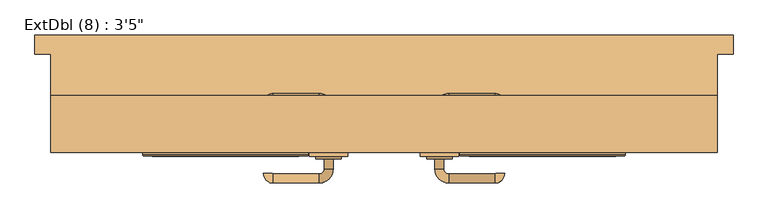
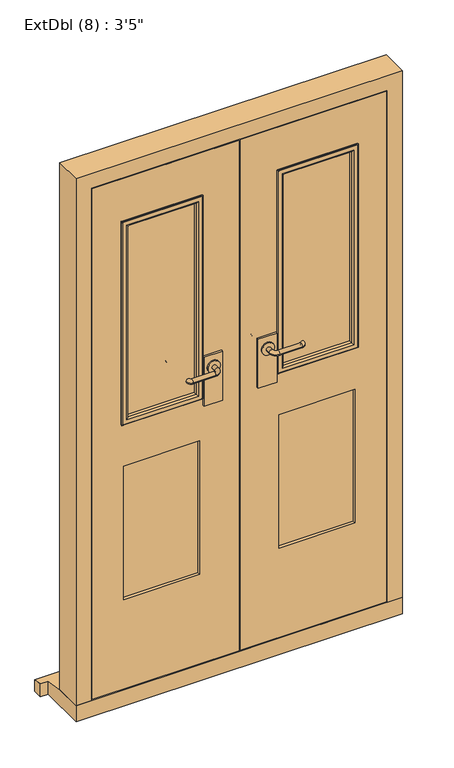
"""IFC4 building model written with IfcOpenShell, lengths in millimetres: door geometry."""

from ifc_helpers import new_model, si_unit, point, frame, frame_2d, origin, place, context, project, spatial, polyline, circle_curve, ellipse_curve, trimmed, segment, composite_curve, outline, extrude, faceted_brep, source, transform, mapped, element, save
from ifc_brep_helpers import plane_surface, cylinder_surface, revolved_surface, advanced_brep


def door_a196e7a2(model_context):
    return source(origin(), model_context, "Body", "SolidModel", [
        extrude(outline(composite_curve([segment(trimmed(circle_curve(frame_2d((1050.0, 86.5)), 20.0), [point((1050.0, 66.5))], [point((1050.0, 106.5))], False, "CARTESIAN"), True, "CONTINUOUS"), segment(trimmed(circle_curve(frame_2d((1050.0, 86.5)), 20.0), [point((1050.0, 106.5))], [point((1050.0, 66.5))], False, "CARTESIAN"), True, "CONTINUOUS")], self_intersect=False)), frame((0.0, -50.2929895, 0.0), z_axis=(0.0, 1.0, 0.0), x_axis=(0.0, 0.0, 1.0)), (0.0, 0.0, 1.0), 4.5929895),
        advanced_brep(
        [(93.5, -50.2929895, 1050.0), (79.5, -50.2929895, 1050.0), (79.5, -65.7, 1050.0), (93.5, -65.7, 1050.0), (101.5, -87.7, 1050.0), (101.5, -73.7, 1050.0), (173.5, -87.7, 1050.0), (173.5, -73.7, 1050.0), (174.5, -72.7, 1050.0), (188.5, -72.7, 1050.0)],
        [
            (0, 1, circle_curve(frame((86.5, -50.2929895, 1050.0), z_axis=(0.0, 1.0, 0.0), x_axis=(-1.0, 0.0, 0.0)), 7.0)),
            (1, 0, circle_curve(frame((86.5, -50.2929895, 1050.0), z_axis=(0.0, 1.0, 0.0), x_axis=(-1.0, 0.0, 0.0)), 7.0)),
            (1, 2),
            (2, 3, circle_curve(frame((86.5, -65.7, 1050.0), z_axis=(0.0, 1.0, 0.0), x_axis=(-1.0, 0.0, 0.0)), 7.0)),
            (3, 0),
            (3, 2, circle_curve(frame((86.5, -65.7, 1050.0), z_axis=(0.0, 1.0, 0.0), x_axis=(-1.0, 0.0, 0.0)), 7.0)),
            (4, 5, circle_curve(frame((101.5, -80.7, 1050.0), z_axis=(-1.0, 0.0, 0.0), x_axis=(0.0, -1.0, 0.0)), 7.0)),
            (5, 3, circle_curve(frame((101.5, -65.7, 1050.0), z_axis=(0.0, 0.0, -1.0), x_axis=(-1.0, 0.0, 0.0)), 8.0)),
            (2, 4, circle_curve(frame((101.5, -65.7, 1050.0), z_axis=(0.0, 0.0, 1.0), x_axis=(-1.0, 0.0, 0.0)), 22.0)),
            (5, 4, circle_curve(frame((101.5, -80.7, 1050.0), z_axis=(-1.0, 0.0, 0.0), x_axis=(0.0, -1.0, 0.0)), 7.0)),
            (4, 6),
            (6, 7, circle_curve(frame((173.5, -80.7, 1050.0), z_axis=(-1.0, 0.0, 0.0), x_axis=(0.0, -1.0, 0.0)), 7.0)),
            (7, 5),
            (7, 6, circle_curve(frame((173.5, -80.7, 1050.0), z_axis=(-1.0, 0.0, 0.0), x_axis=(0.0, -1.0, 0.0)), 7.0)),
            (8, 9, circle_curve(frame((181.5, -72.7, 1050.0), z_axis=(0.0, 1.0, 0.0), x_axis=(1.0, 0.0, 0.0)), 7.0)),
            (9, 8, circle_curve(frame((181.5, -72.7, 1050.0), z_axis=(0.0, 1.0, 0.0), x_axis=(1.0, 0.0, 0.0)), 7.0)),
            (8, 7, circle_curve(frame((173.5, -72.7, 1050.0), z_axis=(0.0, 0.0, -1.0), x_axis=(0.0, -1.0, 0.0)), 1.0)),
            (6, 9, circle_curve(frame((173.5, -72.7, 1050.0), z_axis=(0.0, 0.0, 1.0), x_axis=(0.0, -1.0, 0.0)), 15.0)),
        ],
        [
            plane_surface(frame((86.5, -50.2929895, 1050.0), z_axis=(0.0, 1.0, 0.0), x_axis=(0.0, 0.0, 1.0))),
            cylinder_surface(frame((86.5, -50.2929895, 1050.0), z_axis=(0.0, 1.0, 0.0), x_axis=(-1.0, 0.0, 0.0)), 7.0),
            revolved_surface(trimmed(ellipse_curve(frame((86.5, -65.7, 1050.0), z_axis=(0.0, -1.0, 0.0), x_axis=(-1.0, 0.0, 0.0)), 7.0, 7.0), [point((93.5, -65.7, 1050.0))], [point((79.5, -65.7, 1050.0))], True, "CARTESIAN"), (101.5, -65.7, 1050.0), (0.0, 0.0, -1.0)),
            revolved_surface(trimmed(ellipse_curve(frame((86.5, -65.7, 1050.0), z_axis=(0.0, -1.0, 0.0), x_axis=(-1.0, 0.0, 0.0)), 7.0, 7.0), [point((79.5, -65.7, 1050.0))], [point((93.5, -65.7, 1050.0))], True, "CARTESIAN"), (101.5, -65.7, 1050.0), (0.0, 0.0, -1.0)),
            cylinder_surface(frame((101.5, -80.7, 1050.0), z_axis=(-1.0, 0.0, 0.0), x_axis=(0.0, -1.0, 0.0)), 7.0),
            plane_surface(frame((181.5, -72.7, 1050.0), z_axis=(0.0, 1.0, 0.0), x_axis=(0.0, 0.0, 1.0))),
            revolved_surface(trimmed(ellipse_curve(frame((173.5, -80.7, 1050.0), z_axis=(1.0, 0.0, 0.0), x_axis=(0.0, -1.0, 0.0)), 7.0, 7.0), [point((173.5, -73.7, 1050.0))], [point((173.5, -87.7, 1050.0))], True, "CARTESIAN"), (173.5, -72.7, 1050.0), (0.0, 0.0, -1.0)),
            revolved_surface(trimmed(ellipse_curve(frame((173.5, -80.7, 1050.0), z_axis=(1.0, 0.0, 0.0), x_axis=(0.0, -1.0, 0.0)), 7.0, 7.0), [point((173.5, -87.7, 1050.0))], [point((173.5, -73.7, 1050.0))], True, "CARTESIAN"), (173.5, -72.7, 1050.0), (0.0, 0.0, -1.0)),
        ],
        [
            (0, [[1, 2]]),
            (1, [[3, 4, 5, -2]]),
            (1, [[-5, 6, -3, -1]]),
            (2, [[7, 8, -4, 9]]),
            (3, [[10, -9, -6, -8]]),
            (4, [[11, 12, 13, -7]]),
            (4, [[-13, 14, -11, -10]]),
            (5, [[15, 16]]),
            (6, [[-15, 17, -12, 18]]),
            (7, [[-16, -18, -14, -17]]),
        ],
    ),
        extrude(outline(polyline([(116.5, -39.7), (116.5, -45.7), (56.5, -45.7), (56.5, -39.7), (116.5, -39.7)])), frame((0.0, 0.0, 925.0), z_axis=(0.0, 0.0, 1.0), x_axis=(1.0, 0.0, 0.0)), (0.0, 0.0, 1.0), 165.0),
        extrude(outline(composite_curve([segment(trimmed(circle_curve(frame_2d((1050.0, -86.5)), 20.0), [point((1050.0, -66.5))], [point((1050.0, -106.5))], False, "CARTESIAN"), True, "CONTINUOUS"), segment(trimmed(circle_curve(frame_2d((1050.0, -86.5)), 20.0), [point((1050.0, -106.5))], [point((1050.0, -66.5))], False, "CARTESIAN"), True, "CONTINUOUS")], self_intersect=False)), frame((0.0, -50.2929895, 0.0), z_axis=(0.0, 1.0, 0.0), x_axis=(0.0, 0.0, 1.0)), (0.0, 0.0, 1.0), 4.5929895),
        advanced_brep(
        [(-93.5, -50.2929895, 1050.0), (-79.5, -50.2929895, 1050.0), (-93.5, -65.7, 1050.0), (-79.5, -65.7, 1050.0), (-101.5, -87.7, 1050.0), (-101.5, -73.7, 1050.0), (-173.5, -73.7, 1050.0), (-173.5, -87.7, 1050.0), (-174.5, -72.7, 1050.0), (-188.5, -72.7, 1050.0)],
        [
            (0, 1, circle_curve(frame((-86.5, -50.2929895, 1050.0), z_axis=(0.0, 1.0, 0.0), x_axis=(1.0, 0.0, 0.0)), 7.0)),
            (1, 0, circle_curve(frame((-86.5, -50.2929895, 1050.0), z_axis=(0.0, 1.0, 0.0), x_axis=(1.0, 0.0, 0.0)), 7.0)),
            (0, 2),
            (2, 3, circle_curve(frame((-86.5, -65.7, 1050.0), z_axis=(0.0, 1.0, 0.0), x_axis=(1.0, 0.0, 0.0)), 7.0)),
            (3, 1),
            (3, 2, circle_curve(frame((-86.5, -65.7, 1050.0), z_axis=(0.0, 1.0, 0.0), x_axis=(1.0, 0.0, 0.0)), 7.0)),
            (4, 3, circle_curve(frame((-101.5, -65.7, 1050.0), z_axis=(0.0, 0.0, 1.0), x_axis=(1.0, 0.0, 0.0)), 22.0)),
            (2, 5, circle_curve(frame((-101.5, -65.7, 1050.0), z_axis=(0.0, 0.0, -1.0), x_axis=(1.0, 0.0, 0.0)), 8.0)),
            (5, 4, circle_curve(frame((-101.5, -80.7, 1050.0), z_axis=(1.0, 0.0, 0.0), x_axis=(0.0, -1.0, 0.0)), 7.0)),
            (4, 5, circle_curve(frame((-101.5, -80.7, 1050.0), z_axis=(1.0, 0.0, 0.0), x_axis=(0.0, -1.0, 0.0)), 7.0)),
            (5, 6),
            (6, 7, circle_curve(frame((-173.5, -80.7, 1050.0), z_axis=(1.0, 0.0, 0.0), x_axis=(0.0, -1.0, 0.0)), 7.0)),
            (7, 4),
            (7, 6, circle_curve(frame((-173.5, -80.7, 1050.0), z_axis=(1.0, 0.0, 0.0), x_axis=(0.0, -1.0, 0.0)), 7.0)),
            (8, 9, circle_curve(frame((-181.5, -72.7, 1050.0), z_axis=(0.0, 1.0, 0.0), x_axis=(-1.0, 0.0, 0.0)), 7.0)),
            (9, 8, circle_curve(frame((-181.5, -72.7, 1050.0), z_axis=(0.0, 1.0, 0.0), x_axis=(-1.0, 0.0, 0.0)), 7.0)),
            (9, 7, circle_curve(frame((-173.5, -72.7, 1050.0), z_axis=(0.0, 0.0, 1.0), x_axis=(0.0, -1.0, 0.0)), 15.0)),
            (6, 8, circle_curve(frame((-173.5, -72.7, 1050.0), z_axis=(0.0, 0.0, -1.0), x_axis=(0.0, -1.0, 0.0)), 1.0)),
        ],
        [
            plane_surface(frame((-86.5, -50.2929895, 1050.0), z_axis=(0.0, 1.0, 0.0), x_axis=(0.0, 0.0, 1.0))),
            cylinder_surface(frame((-86.5, -50.2929895, 1050.0), z_axis=(0.0, 1.0, 0.0), x_axis=(1.0, 0.0, 0.0)), 7.0),
            revolved_surface(trimmed(ellipse_curve(frame((-86.5, -65.7, 1050.0), z_axis=(0.0, 1.0, 0.0), x_axis=(1.0, 0.0, 0.0)), 7.0, 7.0), [point((-93.5, -65.7, 1050.0))], [point((-79.5, -65.7, 1050.0))], True, "CARTESIAN"), (-101.5, -65.7, 1050.0), (0.0, 0.0, -1.0)),
            revolved_surface(trimmed(ellipse_curve(frame((-86.5, -65.7, 1050.0), z_axis=(0.0, 1.0, 0.0), x_axis=(1.0, 0.0, 0.0)), 7.0, 7.0), [point((-79.5, -65.7, 1050.0))], [point((-93.5, -65.7, 1050.0))], True, "CARTESIAN"), (-101.5, -65.7, 1050.0), (0.0, 0.0, -1.0)),
            cylinder_surface(frame((-101.5, -80.7, 1050.0), z_axis=(1.0, 0.0, 0.0), x_axis=(0.0, -1.0, 0.0)), 7.0),
            plane_surface(frame((-181.5, -72.7, 1050.0), z_axis=(0.0, 1.0, 0.0), x_axis=(0.0, 0.0, 1.0))),
            revolved_surface(trimmed(ellipse_curve(frame((-173.5, -80.7, 1050.0), z_axis=(1.0, 0.0, 0.0), x_axis=(0.0, -1.0, 0.0)), 7.0, 7.0), [point((-173.5, -73.7, 1050.0))], [point((-173.5, -87.7, 1050.0))], True, "CARTESIAN"), (-173.5, -72.7, 1050.0), (0.0, 0.0, -1.0)),
            revolved_surface(trimmed(ellipse_curve(frame((-173.5, -80.7, 1050.0), z_axis=(1.0, 0.0, 0.0), x_axis=(0.0, -1.0, 0.0)), 7.0, 7.0), [point((-173.5, -87.7, 1050.0))], [point((-173.5, -73.7, 1050.0))], True, "CARTESIAN"), (-173.5, -72.7, 1050.0), (0.0, 0.0, -1.0)),
        ],
        [
            (0, [[1, 2]]),
            (1, [[-1, 3, 4, 5]]),
            (1, [[-2, -5, 6, -3]]),
            (2, [[7, -4, 8, 9]]),
            (3, [[-8, -6, -7, 10]]),
            (4, [[-9, 11, 12, 13]]),
            (4, [[-10, -13, 14, -11]]),
            (5, [[15, 16]]),
            (6, [[17, -12, 18, -16]]),
            (7, [[-18, -14, -17, -15]]),
        ],
    ),
        extrude(outline(polyline([(-116.5, -39.7), (-56.5, -39.7), (-56.5, -45.7), (-116.5, -45.7), (-116.5, -39.7)])), frame((0.0, 0.0, 925.0), z_axis=(0.0, 0.0, 1.0), x_axis=(1.0, 0.0, 0.0)), (0.0, 0.0, 1.0), 165.0),
        extrude(outline(composite_curve([segment(trimmed(circle_curve(frame_2d((1050.0, -86.5)), 20.0), [point((1050.0, -66.5))], [point((1050.0, -106.5))], False, "CARTESIAN"), True, "CONTINUOUS"), segment(trimmed(circle_curve(frame_2d((1050.0, -86.5)), 20.0), [point((1050.0, -106.5))], [point((1050.0, -66.5))], False, "CARTESIAN"), True, "CONTINUOUS")], self_intersect=False)), frame((0.0, 10.3, 0.0), z_axis=(0.0, 1.0, 0.0), x_axis=(0.0, 0.0, 1.0)), (0.0, 0.0, 1.0), 4.5929895),
        advanced_brep(
        [(-93.5, 14.8929895, 1050.0), (-79.5, 14.8929895, 1050.0), (-79.5, 30.3, 1050.0), (-93.5, 30.3, 1050.0), (-101.5, 52.3, 1050.0), (-101.5, 38.3, 1050.0), (-173.5, 52.3, 1050.0), (-173.5, 38.3, 1050.0), (-174.5, 37.3, 1050.0), (-188.5, 37.3, 1050.0)],
        [
            (0, 1, circle_curve(frame((-86.5, 14.8929895, 1050.0), z_axis=(0.0, -1.0, 0.0), x_axis=(1.0, 0.0, 0.0)), 7.0)),
            (1, 0, circle_curve(frame((-86.5, 14.8929895, 1050.0), z_axis=(0.0, -1.0, 0.0), x_axis=(1.0, 0.0, 0.0)), 7.0)),
            (1, 2),
            (2, 3, circle_curve(frame((-86.5, 30.3, 1050.0), z_axis=(0.0, -1.0, 0.0), x_axis=(1.0, 0.0, 0.0)), 7.0)),
            (3, 0),
            (3, 2, circle_curve(frame((-86.5, 30.3, 1050.0), z_axis=(0.0, -1.0, 0.0), x_axis=(1.0, 0.0, 0.0)), 7.0)),
            (4, 5, circle_curve(frame((-101.5, 45.3, 1050.0), z_axis=(1.0, 0.0, 0.0), x_axis=(0.0, 1.0, 0.0)), 7.0)),
            (5, 3, circle_curve(frame((-101.5, 30.3, 1050.0), z_axis=(0.0, 0.0, -1.0), x_axis=(1.0, 0.0, 0.0)), 8.0)),
            (2, 4, circle_curve(frame((-101.5, 30.3, 1050.0), z_axis=(0.0, 0.0, 1.0), x_axis=(1.0, 0.0, 0.0)), 22.0)),
            (5, 4, circle_curve(frame((-101.5, 45.3, 1050.0), z_axis=(1.0, 0.0, 0.0), x_axis=(0.0, 1.0, 0.0)), 7.0)),
            (4, 6),
            (6, 7, circle_curve(frame((-173.5, 45.3, 1050.0), z_axis=(1.0, 0.0, 0.0), x_axis=(0.0, 1.0, 0.0)), 7.0)),
            (7, 5),
            (7, 6, circle_curve(frame((-173.5, 45.3, 1050.0), z_axis=(1.0, 0.0, 0.0), x_axis=(0.0, 1.0, 0.0)), 7.0)),
            (8, 9, circle_curve(frame((-181.5, 37.3, 1050.0), z_axis=(0.0, -1.0, 0.0), x_axis=(-1.0, 0.0, 0.0)), 7.0)),
            (9, 8, circle_curve(frame((-181.5, 37.3, 1050.0), z_axis=(0.0, -1.0, 0.0), x_axis=(-1.0, 0.0, 0.0)), 7.0)),
            (8, 7, circle_curve(frame((-173.5, 37.3, 1050.0), z_axis=(0.0, 0.0, -1.0), x_axis=(0.0, 1.0, 0.0)), 1.0)),
            (6, 9, circle_curve(frame((-173.5, 37.3, 1050.0), z_axis=(0.0, 0.0, 1.0), x_axis=(0.0, 1.0, 0.0)), 15.0)),
        ],
        [
            plane_surface(frame((-86.5, 14.8929895, 1050.0), z_axis=(0.0, -1.0, 0.0), x_axis=(0.0, 0.0, 1.0))),
            cylinder_surface(frame((-86.5, 14.8929895, 1050.0), z_axis=(0.0, -1.0, 0.0), x_axis=(1.0, 0.0, 0.0)), 7.0),
            revolved_surface(trimmed(ellipse_curve(frame((-86.5, 30.3, 1050.0), z_axis=(0.0, 1.0, 0.0), x_axis=(1.0, 0.0, 0.0)), 7.0, 7.0), [point((-93.5, 30.3, 1050.0))], [point((-79.5, 30.3, 1050.0))], True, "CARTESIAN"), (-101.5, 30.3, 1050.0), (0.0, 0.0, -1.0)),
            revolved_surface(trimmed(ellipse_curve(frame((-86.5, 30.3, 1050.0), z_axis=(0.0, 1.0, 0.0), x_axis=(1.0, 0.0, 0.0)), 7.0, 7.0), [point((-79.5, 30.3, 1050.0))], [point((-93.5, 30.3, 1050.0))], True, "CARTESIAN"), (-101.5, 30.3, 1050.0), (0.0, 0.0, -1.0)),
            cylinder_surface(frame((-101.5, 45.3, 1050.0), z_axis=(1.0, 0.0, 0.0), x_axis=(0.0, 1.0, 0.0)), 7.0),
            plane_surface(frame((-181.5, 37.3, 1050.0), z_axis=(0.0, -1.0, 0.0), x_axis=(0.0, 0.0, 1.0))),
            revolved_surface(trimmed(ellipse_curve(frame((-173.5, 45.3, 1050.0), z_axis=(-1.0, 0.0, 0.0), x_axis=(0.0, 1.0, 0.0)), 7.0, 7.0), [point((-173.5, 38.3, 1050.0))], [point((-173.5, 52.3, 1050.0))], True, "CARTESIAN"), (-173.5, 37.3, 1050.0), (0.0, 0.0, -1.0)),
            revolved_surface(trimmed(ellipse_curve(frame((-173.5, 45.3, 1050.0), z_axis=(-1.0, 0.0, 0.0), x_axis=(0.0, 1.0, 0.0)), 7.0, 7.0), [point((-173.5, 52.3, 1050.0))], [point((-173.5, 38.3, 1050.0))], True, "CARTESIAN"), (-173.5, 37.3, 1050.0), (0.0, 0.0, -1.0)),
        ],
        [
            (0, [[1, 2]]),
            (1, [[3, 4, 5, -2]]),
            (1, [[-5, 6, -3, -1]]),
            (2, [[7, 8, -4, 9]]),
            (3, [[10, -9, -6, -8]]),
            (4, [[11, 12, 13, -7]]),
            (4, [[-13, 14, -11, -10]]),
            (5, [[15, 16]]),
            (6, [[-15, 17, -12, 18]]),
            (7, [[-16, -18, -14, -17]]),
        ],
    ),
        extrude(outline(polyline([(-116.5, 4.3), (-116.5, 10.3), (-56.5, 10.3), (-56.5, 4.3), (-116.5, 4.3)])), frame((0.0, 0.0, 925.0), z_axis=(0.0, 0.0, 1.0), x_axis=(1.0, 0.0, 0.0)), (0.0, 0.0, 1.0), 165.0),
        extrude(outline(composite_curve([segment(trimmed(circle_curve(frame_2d((1050.0, 86.5)), 20.0), [point((1050.0, 66.5))], [point((1050.0, 106.5))], False, "CARTESIAN"), True, "CONTINUOUS"), segment(trimmed(circle_curve(frame_2d((1050.0, 86.5)), 20.0), [point((1050.0, 106.5))], [point((1050.0, 66.5))], False, "CARTESIAN"), True, "CONTINUOUS")], self_intersect=False)), frame((0.0, 10.3, 0.0), z_axis=(0.0, 1.0, 0.0), x_axis=(0.0, 0.0, 1.0)), (0.0, 0.0, 1.0), 4.5929895),
        advanced_brep(
        [(93.5, 14.8929895, 1050.0), (79.5, 14.8929895, 1050.0), (93.5, 30.3, 1050.0), (79.5, 30.3, 1050.0), (101.5, 52.3, 1050.0), (101.5, 38.3, 1050.0), (173.5, 38.3, 1050.0), (173.5, 52.3, 1050.0), (174.5, 37.3, 1050.0), (188.5, 37.3, 1050.0)],
        [
            (0, 1, circle_curve(frame((86.5, 14.8929895, 1050.0), z_axis=(0.0, -1.0, 0.0), x_axis=(-1.0, 0.0, 0.0)), 7.0)),
            (1, 0, circle_curve(frame((86.5, 14.8929895, 1050.0), z_axis=(0.0, -1.0, 0.0), x_axis=(-1.0, 0.0, 0.0)), 7.0)),
            (0, 2),
            (2, 3, circle_curve(frame((86.5, 30.3, 1050.0), z_axis=(0.0, -1.0, 0.0), x_axis=(-1.0, 0.0, 0.0)), 7.0)),
            (3, 1),
            (3, 2, circle_curve(frame((86.5, 30.3, 1050.0), z_axis=(0.0, -1.0, 0.0), x_axis=(-1.0, 0.0, 0.0)), 7.0)),
            (4, 3, circle_curve(frame((101.5, 30.3, 1050.0), z_axis=(0.0, 0.0, 1.0), x_axis=(-1.0, 0.0, 0.0)), 22.0)),
            (2, 5, circle_curve(frame((101.5, 30.3, 1050.0), z_axis=(0.0, 0.0, -1.0), x_axis=(-1.0, 0.0, 0.0)), 8.0)),
            (5, 4, circle_curve(frame((101.5, 45.3, 1050.0), z_axis=(-1.0, 0.0, 0.0), x_axis=(0.0, 1.0, 0.0)), 7.0)),
            (4, 5, circle_curve(frame((101.5, 45.3, 1050.0), z_axis=(-1.0, 0.0, 0.0), x_axis=(0.0, 1.0, 0.0)), 7.0)),
            (5, 6),
            (6, 7, circle_curve(frame((173.5, 45.3, 1050.0), z_axis=(-1.0, 0.0, 0.0), x_axis=(0.0, 1.0, 0.0)), 7.0)),
            (7, 4),
            (7, 6, circle_curve(frame((173.5, 45.3, 1050.0), z_axis=(-1.0, 0.0, 0.0), x_axis=(0.0, 1.0, 0.0)), 7.0)),
            (8, 9, circle_curve(frame((181.5, 37.3, 1050.0), z_axis=(0.0, -1.0, 0.0), x_axis=(1.0, 0.0, 0.0)), 7.0)),
            (9, 8, circle_curve(frame((181.5, 37.3, 1050.0), z_axis=(0.0, -1.0, 0.0), x_axis=(1.0, 0.0, 0.0)), 7.0)),
            (9, 7, circle_curve(frame((173.5, 37.3, 1050.0), z_axis=(0.0, 0.0, 1.0), x_axis=(0.0, 1.0, 0.0)), 15.0)),
            (6, 8, circle_curve(frame((173.5, 37.3, 1050.0), z_axis=(0.0, 0.0, -1.0), x_axis=(0.0, 1.0, 0.0)), 1.0)),
        ],
        [
            plane_surface(frame((86.5, 14.8929895, 1050.0), z_axis=(0.0, -1.0, 0.0), x_axis=(0.0, 0.0, 1.0))),
            cylinder_surface(frame((86.5, 14.8929895, 1050.0), z_axis=(0.0, -1.0, 0.0), x_axis=(-1.0, 0.0, 0.0)), 7.0),
            revolved_surface(trimmed(ellipse_curve(frame((86.5, 30.3, 1050.0), z_axis=(0.0, -1.0, 0.0), x_axis=(-1.0, 0.0, 0.0)), 7.0, 7.0), [point((93.5, 30.3, 1050.0))], [point((79.5, 30.3, 1050.0))], True, "CARTESIAN"), (101.5, 30.3, 1050.0), (0.0, 0.0, -1.0)),
            revolved_surface(trimmed(ellipse_curve(frame((86.5, 30.3, 1050.0), z_axis=(0.0, -1.0, 0.0), x_axis=(-1.0, 0.0, 0.0)), 7.0, 7.0), [point((79.5, 30.3, 1050.0))], [point((93.5, 30.3, 1050.0))], True, "CARTESIAN"), (101.5, 30.3, 1050.0), (0.0, 0.0, -1.0)),
            cylinder_surface(frame((101.5, 45.3, 1050.0), z_axis=(-1.0, 0.0, 0.0), x_axis=(0.0, 1.0, 0.0)), 7.0),
            plane_surface(frame((181.5, 37.3, 1050.0), z_axis=(0.0, -1.0, 0.0), x_axis=(0.0, 0.0, 1.0))),
            revolved_surface(trimmed(ellipse_curve(frame((173.5, 45.3, 1050.0), z_axis=(-1.0, 0.0, 0.0), x_axis=(0.0, 1.0, 0.0)), 7.0, 7.0), [point((173.5, 38.3, 1050.0))], [point((173.5, 52.3, 1050.0))], True, "CARTESIAN"), (173.5, 37.3, 1050.0), (0.0, 0.0, -1.0)),
            revolved_surface(trimmed(ellipse_curve(frame((173.5, 45.3, 1050.0), z_axis=(-1.0, 0.0, 0.0), x_axis=(0.0, 1.0, 0.0)), 7.0, 7.0), [point((173.5, 52.3, 1050.0))], [point((173.5, 38.3, 1050.0))], True, "CARTESIAN"), (173.5, 37.3, 1050.0), (0.0, 0.0, -1.0)),
        ],
        [
            (0, [[1, 2]]),
            (1, [[-1, 3, 4, 5]]),
            (1, [[-2, -5, 6, -3]]),
            (2, [[7, -4, 8, 9]]),
            (3, [[-8, -6, -7, 10]]),
            (4, [[-9, 11, 12, 13]]),
            (4, [[-10, -13, 14, -11]]),
            (5, [[15, 16]]),
            (6, [[17, -12, 18, -16]]),
            (7, [[-18, -14, -17, -15]]),
        ],
    ),
        extrude(outline(polyline([(116.5, 4.3), (56.5, 4.3), (56.5, 10.3), (116.5, 10.3), (116.5, 4.3)])), frame((0.0, 0.0, 925.0), z_axis=(0.0, 0.0, 1.0), x_axis=(1.0, 0.0, 0.0)), (0.0, 0.0, 1.0), 165.0),
        faceted_brep([(450.2, 49.3, 54.5), (520.7, 49.3, 54.5), (520.7, -39.7, 54.5), (472.2, -39.7, 54.5), (472.2, 7.3, 54.5), (450.2, 7.3, 54.5), (450.2, 49.3, 1758.3), (-450.2, 49.3, 1758.3), (-450.2, 49.3, 54.5), (-520.7, 49.3, 54.5), (-520.7, 49.3, 1828.8), (520.7, 49.3, 1828.8), (520.7, -39.7, 1828.8), (-520.7, -39.7, 1828.8), (-520.7, -39.7, 54.5), (-472.2, -39.7, 54.5), (-472.2, -39.7, 1780.3), (472.2, -39.7, 1780.3), (472.2, 7.3, 1780.3), (-472.2, 7.3, 1780.3), (-472.2, 7.3, 54.5), (-450.2, 7.3, 54.5), (-450.2, 7.3, 1758.3), (450.2, 7.3, 1758.3)], [[[0, 1, 2, 3, 4, 5]], [[1, 0, 6, 7, 8, 9, 10, 11]], [[2, 1, 11, 12]], [[3, 2, 12, 13, 14, 15, 16, 17]], [[4, 3, 17, 18]], [[5, 4, 18, 19, 20, 21, 22, 23]], [[0, 5, 23, 6]], [[7, 22, 21, 8]], [[8, 21, 20, 15, 14, 9]], [[13, 10, 9, 14]], [[19, 16, 15, 20]], [[12, 11, 10, 13]], [[18, 17, 16, 19]], [[6, 23, 22, 7]]]),
        extrude(outline(polyline([(58.5, 469.2), (1777.3, 469.2), (1777.3, 1.5), (58.5, 1.5), (58.5, 469.2)]), holes=[polyline([(1627.3, 369.2), (958.5, 369.2), (958.5, 126.5), (1627.3, 126.5), (1627.3, 369.2)]), polyline([(808.5, 126.5), (808.5, 369.2), (358.5, 369.2), (358.5, 126.5), (808.5, 126.5)])]), frame((0.0, -39.7, 0.0), z_axis=(0.0, 1.0, 0.0), x_axis=(0.0, 0.0, 1.0)), (0.0, 0.0, 1.0), 44.0),
        extrude(outline(polyline([(58.5, -469.2), (58.5, -1.5), (1777.3, -1.5), (1777.3, -469.2), (58.5, -469.2)]), holes=[polyline([(1627.3, -126.5), (958.5, -126.5), (958.5, -369.2), (1627.3, -369.2), (1627.3, -126.5)]), polyline([(808.5, -369.2), (808.5, -126.5), (358.5, -126.5), (358.5, -369.2), (808.5, -369.2)])]), frame((0.0, -39.7, 0.0), z_axis=(0.0, 1.0, 0.0), x_axis=(0.0, 0.0, 1.0)), (0.0, 0.0, 1.0), 44.0),
        faceted_brep([(545.7, 144.3, 0.0), (545.7, 144.3, 38.5947221), (545.7, 114.3, 43.6174415), (545.7, 114.3, 0.0), (-545.7, 144.3, 38.5947221), (-545.7, 144.3, 0.0), (-545.7, 114.3, 0.0), (-545.7, 114.3, 43.6174415), (520.7, 114.3, 0.0), (520.7, -39.7, 0.0), (-520.7, -39.7, 0.0), (-520.7, 114.3, 0.0), (-520.7, 114.3, 43.6174415), (-520.7, 49.3, 54.5), (520.7, 49.3, 54.5), (520.7, 114.3, 43.6174415), (-520.7, -39.7, 54.5), (520.7, -39.7, 54.5)], [[[0, 1, 2, 3]], [[4, 5, 6, 7]], [[5, 0, 3, 8, 9, 10, 11, 6]], [[1, 0, 5, 4]], [[1, 4, 7, 12, 13, 14, 15, 2]], [[13, 16, 17, 14]], [[16, 10, 9, 17]], [[12, 11, 10, 16, 13]], [[11, 12, 7, 6]], [[8, 15, 14, 17, 9]], [[15, 8, 3, 2]]]),
        extrude(outline(polyline([(126.5, -5.7), (367.6390207, -5.7), (367.6390207, -29.7), (126.5, -29.7), (126.5, -5.7)])), frame((0.0, 0.0, 958.5), z_axis=(0.0, 0.0, 1.0), x_axis=(1.0, 0.0, 0.0)), (0.0, 0.0, 1.0), 668.8),
        extrude(outline(polyline([(-369.2, -5.7), (-126.5, -5.7), (-126.5, -29.7), (-369.2, -29.7), (-369.2, -5.7)])), frame((0.0, 0.0, 958.5), z_axis=(0.0, 0.0, 1.0), x_axis=(1.0, 0.0, 0.0)), (0.0, 0.0, 1.0), 668.8),
        extrude(outline(polyline([(369.2, -29.7), (126.5, -29.7), (126.5, -5.7), (369.2, -5.7), (369.2, -29.7)])), frame((0.0, 0.0, 358.5), z_axis=(0.0, 0.0, 1.0), x_axis=(1.0, 0.0, 0.0)), (0.0, 0.0, 1.0), 450.0),
        extrude(outline(polyline([(-126.5, -29.7), (-369.2, -29.7), (-369.2, -5.7), (-126.5, -5.7), (-126.5, -29.7)])), frame((0.0, 0.0, 358.5), z_axis=(0.0, 0.0, 1.0), x_axis=(1.0, 0.0, 0.0)), (0.0, 0.0, 1.0), 450.0),
        advanced_brep(
        [(118.5, 8.3, 950.5), (118.5, 4.3, 950.5), (118.5, 4.3, 1635.3), (118.5, 8.3, 1635.3), (120.5, 10.3, 952.5), (120.5, 10.3, 1633.3), (138.5, 5.3, 970.5), (133.5, 10.3, 965.5), (133.5, 10.3, 1620.3), (138.5, 5.3, 1615.3), (138.5, -5.7, 970.5), (138.5, -5.7, 1615.3), (126.5, 4.3, 958.5), (126.5, -5.7, 958.5), (126.5, -5.7, 1627.3), (126.5, 4.3, 1627.3), (377.2, 4.3, 1635.3), (377.2, 8.3, 1635.3), (375.2, 10.3, 1633.3), (362.2, 10.3, 1620.3), (357.2, 5.3, 1615.3), (357.2, -5.7, 1615.3), (369.2, -5.7, 1627.3), (369.2, 4.3, 1627.3), (377.2, 4.3, 950.5), (377.2, 8.3, 950.5), (375.2, 10.3, 952.5), (362.2, 10.3, 965.5), (357.2, 5.3, 970.5), (357.2, -5.7, 970.5), (369.2, -5.7, 958.5), (369.2, 4.3, 958.5)],
        [
            (0, 1),
            (1, 2),
            (2, 3),
            (3, 0),
            (4, 0, ellipse_curve(frame((120.5, 8.3, 952.5), z_axis=(-0.7071067811865475, 0.0, 0.7071067811865476), x_axis=(-0.7071067811865476, 0.0, -0.7071067811865475)), 2.8284271, 2.0)),
            (3, 5, ellipse_curve(frame((120.5, 8.3, 1633.3), z_axis=(-0.7071067811865476, 0.0, -0.7071067811865475), x_axis=(0.7071067811865475, 0.0, -0.7071067811865476)), 2.8284271, 2.0)),
            (5, 4),
            (6, 7, ellipse_curve(frame((133.5, 5.3, 965.5), z_axis=(-0.7071067811865475, 0.0, 0.7071067811865476), x_axis=(-0.7071067811865476, 0.0, -0.7071067811865475)), 7.0710678, 5.0)),
            (7, 8),
            (8, 9, ellipse_curve(frame((133.5, 5.3, 1620.3), z_axis=(-0.7071067811865476, 0.0, -0.7071067811865475), x_axis=(0.7071067811865475, 0.0, -0.7071067811865476)), 7.0710678, 5.0)),
            (9, 6),
            (10, 6),
            (9, 11),
            (11, 10),
            (12, 13),
            (13, 14),
            (14, 15),
            (15, 12),
            (2, 16),
            (16, 17),
            (17, 3),
            (17, 18, ellipse_curve(frame((375.2, 8.3, 1633.3), z_axis=(-0.7071067811865475, 0.0, 0.7071067811865475), x_axis=(-0.7071067811865477, 0.0, -0.7071067811865474)), 2.8284271, 2.0)),
            (18, 5),
            (8, 19),
            (19, 20, ellipse_curve(frame((362.2, 5.3, 1620.3), z_axis=(-0.7071067811865475, 0.0, 0.7071067811865475), x_axis=(-0.7071067811865477, 0.0, -0.7071067811865474)), 7.0710678, 5.0)),
            (20, 9),
            (20, 21),
            (21, 11),
            (14, 22),
            (22, 23),
            (23, 15),
            (16, 24),
            (24, 25),
            (25, 17),
            (25, 26, ellipse_curve(frame((375.2, 8.3, 952.5), z_axis=(0.7071067811865475, 0.0, 0.7071067811865475), x_axis=(-0.7071067811865474, 0.0, 0.7071067811865477)), 2.8284271, 2.0)),
            (26, 18),
            (19, 27),
            (27, 28, ellipse_curve(frame((362.2, 5.3, 965.5), z_axis=(0.7071067811865475, 0.0, 0.7071067811865475), x_axis=(-0.7071067811865474, 0.0, 0.7071067811865477)), 7.0710678, 5.0)),
            (28, 20),
            (28, 29),
            (29, 21),
            (22, 30),
            (30, 31),
            (31, 23),
            (24, 1),
            (0, 25),
            (4, 26),
            (7, 27),
            (6, 28),
            (10, 29),
            (13, 30),
            (12, 31),
        ],
        [
            plane_surface(frame((118.5, 4.3, 950.5), z_axis=(-1.0, 0.0, 0.0), x_axis=(0.0, 0.0, 1.0))),
            cylinder_surface(frame((120.5, 8.3, 958.5), z_axis=(0.0, 0.0, -1.0), x_axis=(-1.0, 0.0, 0.0)), 2.0),
            cylinder_surface(frame((133.5, 5.3, 958.5), z_axis=(0.0, 0.0, -1.0), x_axis=(-1.0, 0.0, 0.0)), 5.0),
            plane_surface(frame((138.5, 5.3, 970.5), z_axis=(1.0, 0.0, 0.0), x_axis=(0.0, 0.0, 1.0))),
            plane_surface(frame((126.5, -5.7, 958.5), z_axis=(-1.0, 0.0, 0.0), x_axis=(0.0, 0.0, 1.0))),
            plane_surface(frame((118.5, 4.3, 1635.3), z_axis=(0.0, 0.0, 1.0), x_axis=(1.0, 0.0, 0.0))),
            cylinder_surface(frame((126.5, 8.3, 1633.3), z_axis=(-1.0, 0.0, 0.0), x_axis=(0.0, 0.0, 1.0)), 2.0),
            cylinder_surface(frame((126.5, 5.3, 1620.3), z_axis=(-1.0, 0.0, 0.0), x_axis=(0.0, 0.0, 1.0)), 5.0),
            plane_surface(frame((138.5, 5.3, 1615.3), z_axis=(0.0, 0.0, -1.0), x_axis=(1.0, 0.0, 0.0))),
            plane_surface(frame((126.5, -5.7, 1627.3), z_axis=(0.0, 0.0, 1.0), x_axis=(1.0, 0.0, 0.0))),
            plane_surface(frame((377.2, 4.3, 1635.3), z_axis=(1.0, 0.0, 0.0), x_axis=(0.0, 0.0, -1.0))),
            cylinder_surface(frame((375.2, 8.3, 1627.3), z_axis=(0.0, 0.0, 1.0), x_axis=(1.0, 0.0, 0.0)), 2.0),
            cylinder_surface(frame((362.2, 5.3, 1627.3), z_axis=(0.0, 0.0, 1.0), x_axis=(1.0, 0.0, 0.0)), 5.0),
            plane_surface(frame((357.2, 5.3, 1615.3), z_axis=(-1.0, 0.0, 0.0), x_axis=(0.0, 0.0, -1.0))),
            plane_surface(frame((369.2, -5.7, 1627.3), z_axis=(1.0, 0.0, 0.0), x_axis=(0.0, 0.0, -1.0))),
            plane_surface(frame((377.2, 4.3, 950.5), z_axis=(0.0, 0.0, -1.0), x_axis=(-1.0, 0.0, 0.0))),
            cylinder_surface(frame((369.2, 8.3, 952.5), z_axis=(1.0, 0.0, 0.0), x_axis=(0.0, 0.0, -1.0)), 2.0),
            plane_surface(frame((375.2, 10.3, 952.5), z_axis=(0.0, 1.0, 0.0), x_axis=(-1.0, 0.0, 0.0))),
            cylinder_surface(frame((369.2, 5.3, 965.5), z_axis=(1.0, 0.0, 0.0), x_axis=(0.0, 0.0, -1.0)), 5.0),
            plane_surface(frame((357.2, 5.3, 970.5), z_axis=(0.0, 0.0, 1.0), x_axis=(-1.0, 0.0, 0.0))),
            plane_surface(frame((357.2, -5.7, 970.5), z_axis=(0.0, -1.0, 0.0), x_axis=(-1.0, 0.0, 0.0))),
            plane_surface(frame((369.2, -5.7, 958.5), z_axis=(0.0, 0.0, -1.0), x_axis=(-1.0, 0.0, 0.0))),
            plane_surface(frame((369.2, 4.3, 958.5), z_axis=(0.0, -1.0, 0.0), x_axis=(-1.0, 0.0, 0.0))),
        ],
        [
            (0, [[1, 2, 3, 4]]),
            (1, [[5, -4, 6, 7]]),
            (2, [[8, 9, 10, 11]]),
            (3, [[12, -11, 13, 14]]),
            (4, [[15, 16, 17, 18]]),
            (5, [[-3, 19, 20, 21]]),
            (6, [[-6, -21, 22, 23]]),
            (7, [[-10, 24, 25, 26]]),
            (8, [[-13, -26, 27, 28]]),
            (9, [[-17, 29, 30, 31]]),
            (10, [[-20, 32, 33, 34]]),
            (11, [[-22, -34, 35, 36]]),
            (12, [[-25, 37, 38, 39]]),
            (13, [[-27, -39, 40, 41]]),
            (14, [[-30, 42, 43, 44]]),
            (15, [[-33, 45, -1, 46]]),
            (16, [[-35, -46, -5, 47]]),
            (17, [[-23, -36, -47, -7], [48, -37, -24, -9]]),
            (18, [[-38, -48, -8, 49]]),
            (19, [[-40, -49, -12, 50]]),
            (20, [[51, -42, -29, -16], [-28, -41, -50, -14]]),
            (21, [[-43, -51, -15, 52]]),
            (22, [[-45, -32, -19, -2], [-31, -44, -52, -18]]),
        ],
    ),
        advanced_brep(
        [(369.2, -29.7, 1627.3), (369.2, -39.7, 1627.3), (369.2, -39.7, 958.5), (369.2, -29.7, 958.5), (357.2, -40.7, 1615.3), (357.2, -29.7, 1615.3), (357.2, -29.7, 970.5), (357.2, -40.7, 970.5), (362.2, -45.7, 1620.3), (362.2, -45.7, 965.5), (377.2, -43.7, 1635.3), (375.2, -45.7, 1633.3), (375.2, -45.7, 952.5), (377.2, -43.7, 950.5), (377.2, -39.7, 1635.3), (377.2, -39.7, 950.5), (126.5, -39.7, 958.5), (126.5, -29.7, 958.5), (138.5, -29.7, 970.5), (138.5, -40.7, 970.5), (133.5, -45.7, 965.5), (120.5, -45.7, 952.5), (118.5, -43.7, 950.5), (118.5, -39.7, 950.5), (126.5, -39.7, 1627.3), (126.5, -29.7, 1627.3), (138.5, -29.7, 1615.3), (138.5, -40.7, 1615.3), (133.5, -45.7, 1620.3), (120.5, -45.7, 1633.3), (118.5, -43.7, 1635.3), (118.5, -39.7, 1635.3)],
        [
            (0, 1),
            (1, 2),
            (2, 3),
            (3, 0),
            (4, 5),
            (5, 6),
            (6, 7),
            (7, 4),
            (8, 4, ellipse_curve(frame((362.2, -40.7, 1620.3), z_axis=(0.7071067811865521, 0.0, -0.7071067811865428), x_axis=(0.7071067811865427, 0.0, 0.7071067811865522)), 7.0710678, 5.0)),
            (7, 9, ellipse_curve(frame((362.2, -40.7, 965.5), z_axis=(0.7071067811865431, 0.0, 0.7071067811865518), x_axis=(-0.7071067811865516, 0.0, 0.7071067811865435)), 7.0710678, 5.0)),
            (9, 8),
            (10, 11, ellipse_curve(frame((375.2, -43.7, 1633.3), z_axis=(0.7071067811865521, 0.0, -0.7071067811865428), x_axis=(0.7071067811865427, 0.0, 0.7071067811865522)), 2.8284271, 2.0)),
            (11, 12),
            (12, 13, ellipse_curve(frame((375.2, -43.7, 952.5), z_axis=(0.7071067811865431, 0.0, 0.7071067811865518), x_axis=(-0.7071067811865516, 0.0, 0.7071067811865435)), 2.8284271, 2.0)),
            (13, 10),
            (14, 10),
            (13, 15),
            (15, 14),
            (2, 16),
            (16, 17),
            (17, 3),
            (6, 18),
            (18, 19),
            (19, 7),
            (19, 20, ellipse_curve(frame((133.5, -40.7, 965.5), z_axis=(0.7071067811865519, 0.0, -0.7071067811865431), x_axis=(0.7071067811865431, 0.0, 0.7071067811865518)), 7.0710678, 5.0)),
            (20, 9),
            (12, 21),
            (21, 22, ellipse_curve(frame((120.5, -43.7, 952.5), z_axis=(0.7071067811865519, 0.0, -0.7071067811865431), x_axis=(0.7071067811865431, 0.0, 0.7071067811865518)), 2.8284271, 2.0)),
            (22, 13),
            (22, 23),
            (23, 15),
            (16, 24),
            (24, 25),
            (25, 17),
            (18, 26),
            (26, 27),
            (27, 19),
            (27, 28, ellipse_curve(frame((133.5, -40.7, 1620.3), z_axis=(-0.7071067811865428, 0.0, -0.7071067811865521), x_axis=(0.707106781186552, 0.0, -0.7071067811865431)), 7.0710678, 5.0)),
            (28, 20),
            (21, 29),
            (29, 30, ellipse_curve(frame((120.5, -43.7, 1633.3), z_axis=(-0.7071067811865428, 0.0, -0.7071067811865521), x_axis=(0.707106781186552, 0.0, -0.7071067811865431)), 2.8284271, 2.0)),
            (30, 22),
            (30, 31),
            (31, 23),
            (31, 14),
            (1, 24),
            (0, 25),
            (5, 26),
            (4, 27),
            (8, 28),
            (11, 29),
            (10, 30),
        ],
        [
            plane_surface(frame((369.2, -39.7, 1627.3), z_axis=(1.0, 0.0, 0.0), x_axis=(0.0, 0.0, -1.0))),
            plane_surface(frame((357.2, -29.7, 1615.3), z_axis=(-1.0, 0.0, 0.0), x_axis=(0.0, 0.0, -1.0))),
            cylinder_surface(frame((362.2, -40.7, 1627.3), z_axis=(0.0, 0.0, 1.0), x_axis=(1.0, 0.0, 0.0)), 5.0),
            cylinder_surface(frame((375.2, -43.7, 1627.3), z_axis=(0.0, 0.0, 1.0), x_axis=(1.0, 0.0, 0.0)), 2.0),
            plane_surface(frame((377.2, -43.7, 1635.3), z_axis=(1.0, 0.0, 0.0), x_axis=(0.0, 0.0, -1.0))),
            plane_surface(frame((369.2, -39.7, 958.5), z_axis=(0.0, 0.0, -1.0), x_axis=(-1.0, 0.0, 0.0))),
            plane_surface(frame((357.2, -29.7, 970.5), z_axis=(0.0, 0.0, 1.0), x_axis=(-1.0, 0.0, 0.0))),
            cylinder_surface(frame((369.2, -40.7, 965.5), z_axis=(1.0, 0.0, 0.0), x_axis=(0.0, 0.0, -1.0)), 5.0),
            cylinder_surface(frame((369.2, -43.7, 952.5), z_axis=(1.0, 0.0, 0.0), x_axis=(0.0, 0.0, -1.0)), 2.0),
            plane_surface(frame((377.2, -43.7, 950.5), z_axis=(0.0, 0.0, -1.0), x_axis=(-1.0, 0.0, 0.0))),
            plane_surface(frame((126.5, -39.7, 958.5), z_axis=(-1.0, 0.0, 0.0), x_axis=(0.0, 0.0, 1.0))),
            plane_surface(frame((138.5, -29.7, 970.5), z_axis=(1.0, 0.0, 0.0), x_axis=(0.0, 0.0, 1.0))),
            cylinder_surface(frame((133.5, -40.7, 958.5), z_axis=(0.0, 0.0, -1.0), x_axis=(-1.0, 0.0, 0.0)), 5.0),
            cylinder_surface(frame((120.5, -43.7, 958.5), z_axis=(0.0, 0.0, -1.0), x_axis=(-1.0, 0.0, 0.0)), 2.0),
            plane_surface(frame((118.5, -43.7, 950.5), z_axis=(-1.0, 0.0, 0.0), x_axis=(0.0, 0.0, 1.0))),
            plane_surface(frame((118.5, -39.7, 1635.3), z_axis=(0.0, 1.0, 0.0), x_axis=(1.0, 0.0, 0.0))),
            plane_surface(frame((126.5, -39.7, 1627.3), z_axis=(0.0, 0.0, 1.0), x_axis=(1.0, 0.0, 0.0))),
            plane_surface(frame((126.5, -29.7, 1627.3), z_axis=(0.0, 1.0, 0.0), x_axis=(1.0, 0.0, 0.0))),
            plane_surface(frame((138.5, -29.7, 1615.3), z_axis=(0.0, 0.0, -1.0), x_axis=(1.0, 0.0, 0.0))),
            cylinder_surface(frame((126.5, -40.7, 1620.3), z_axis=(-1.0, 0.0, 0.0), x_axis=(0.0, 0.0, 1.0)), 5.0),
            plane_surface(frame((133.5, -45.7, 1620.3), z_axis=(0.0, -1.0, 0.0), x_axis=(1.0, 0.0, 0.0))),
            cylinder_surface(frame((126.5, -43.7, 1633.3), z_axis=(-1.0, 0.0, 0.0), x_axis=(0.0, 0.0, 1.0)), 2.0),
            plane_surface(frame((118.5, -43.7, 1635.3), z_axis=(0.0, 0.0, 1.0), x_axis=(1.0, 0.0, 0.0))),
        ],
        [
            (0, [[1, 2, 3, 4]]),
            (1, [[5, 6, 7, 8]]),
            (2, [[9, -8, 10, 11]]),
            (3, [[12, 13, 14, 15]]),
            (4, [[16, -15, 17, 18]]),
            (5, [[-3, 19, 20, 21]]),
            (6, [[-7, 22, 23, 24]]),
            (7, [[-10, -24, 25, 26]]),
            (8, [[-14, 27, 28, 29]]),
            (9, [[-17, -29, 30, 31]]),
            (10, [[-20, 32, 33, 34]]),
            (11, [[-23, 35, 36, 37]]),
            (12, [[-25, -37, 38, 39]]),
            (13, [[-28, 40, 41, 42]]),
            (14, [[-30, -42, 43, 44]]),
            (15, [[-31, -44, 45, -18], [46, -32, -19, -2]]),
            (16, [[-33, -46, -1, 47]]),
            (17, [[-21, -34, -47, -4], [48, -35, -22, -6]]),
            (18, [[-36, -48, -5, 49]]),
            (19, [[-38, -49, -9, 50]]),
            (20, [[51, -40, -27, -13], [-26, -39, -50, -11]]),
            (21, [[-41, -51, -12, 52]]),
            (22, [[-43, -52, -16, -45]]),
        ],
    ),
        advanced_brep(
        [(-126.5, -29.7, 1627.3), (-126.5, -39.7, 1627.3), (-126.5, -39.7, 958.5), (-126.5, -29.7, 958.5), (-138.5, -40.7, 1615.3), (-138.5, -29.7, 1615.3), (-138.5, -29.7, 970.5), (-138.5, -40.7, 970.5), (-133.5, -45.7, 1620.3), (-133.5, -45.7, 965.5), (-118.5, -43.7, 1635.3), (-120.5, -45.7, 1633.3), (-120.5, -45.7, 952.5), (-118.5, -43.7, 950.5), (-118.5, -39.7, 1635.3), (-118.5, -39.7, 950.5), (-369.2, -39.7, 958.5), (-369.2, -29.7, 958.5), (-357.2, -29.7, 970.5), (-357.2, -40.7, 970.5), (-362.2, -45.7, 965.5), (-375.2, -45.7, 952.5), (-377.2, -43.7, 950.5), (-377.2, -39.7, 950.5), (-369.2, -39.7, 1627.3), (-369.2, -29.7, 1627.3), (-357.2, -29.7, 1615.3), (-357.2, -40.7, 1615.3), (-362.2, -45.7, 1620.3), (-375.2, -45.7, 1633.3), (-377.2, -43.7, 1635.3), (-377.2, -39.7, 1635.3)],
        [
            (0, 1),
            (1, 2),
            (2, 3),
            (3, 0),
            (4, 5),
            (5, 6),
            (6, 7),
            (7, 4),
            (8, 4, ellipse_curve(frame((-133.5, -40.7, 1620.3), z_axis=(0.7071067811865475, 0.0, -0.7071067811865475), x_axis=(0.7071067811865474, 0.0, 0.7071067811865476)), 7.0710678, 5.0)),
            (7, 9, ellipse_curve(frame((-133.5, -40.7, 965.5), z_axis=(0.7071067811865475, 0.0, 0.7071067811865475), x_axis=(-0.7071067811865474, 0.0, 0.7071067811865476)), 7.0710678, 5.0)),
            (9, 8),
            (10, 11, ellipse_curve(frame((-120.5, -43.7, 1633.3), z_axis=(0.7071067811865475, 0.0, -0.7071067811865475), x_axis=(0.7071067811865474, 0.0, 0.7071067811865476)), 2.8284271, 2.0)),
            (11, 12),
            (12, 13, ellipse_curve(frame((-120.5, -43.7, 952.5), z_axis=(0.7071067811865475, 0.0, 0.7071067811865475), x_axis=(-0.7071067811865474, 0.0, 0.7071067811865476)), 2.8284271, 2.0)),
            (13, 10),
            (14, 10),
            (13, 15),
            (15, 14),
            (2, 16),
            (16, 17),
            (17, 3),
            (6, 18),
            (18, 19),
            (19, 7),
            (19, 20, ellipse_curve(frame((-362.2, -40.7, 965.5), z_axis=(0.7071067811865475, 0.0, -0.7071067811865475), x_axis=(0.7071067811865476, 0.0, 0.7071067811865474)), 7.0710678, 5.0)),
            (20, 9),
            (12, 21),
            (21, 22, ellipse_curve(frame((-375.2, -43.7, 952.5), z_axis=(0.7071067811865475, 0.0, -0.7071067811865475), x_axis=(0.7071067811865476, 0.0, 0.7071067811865474)), 2.8284271, 2.0)),
            (22, 13),
            (22, 23),
            (23, 15),
            (16, 24),
            (24, 25),
            (25, 17),
            (18, 26),
            (26, 27),
            (27, 19),
            (27, 28, ellipse_curve(frame((-362.2, -40.7, 1620.3), z_axis=(-0.7071067811865475, 0.0, -0.7071067811865475), x_axis=(0.7071067811865474, 0.0, -0.7071067811865476)), 7.0710678, 5.0)),
            (28, 20),
            (21, 29),
            (29, 30, ellipse_curve(frame((-375.2, -43.7, 1633.3), z_axis=(-0.7071067811865475, 0.0, -0.7071067811865475), x_axis=(0.7071067811865474, 0.0, -0.7071067811865476)), 2.8284271, 2.0)),
            (30, 22),
            (30, 31),
            (31, 23),
            (31, 14),
            (1, 24),
            (0, 25),
            (5, 26),
            (4, 27),
            (8, 28),
            (11, 29),
            (10, 30),
        ],
        [
            plane_surface(frame((-126.5, -39.7, 1627.3), z_axis=(1.0, 0.0, 0.0), x_axis=(0.0, 0.0, -1.0))),
            plane_surface(frame((-138.5, -29.7, 1615.3), z_axis=(-1.0, 0.0, 0.0), x_axis=(0.0, 0.0, -1.0))),
            cylinder_surface(frame((-133.5, -40.7, 1627.3), z_axis=(0.0, 0.0, 1.0), x_axis=(1.0, 0.0, 0.0)), 5.0),
            cylinder_surface(frame((-120.5, -43.7, 1627.3), z_axis=(0.0, 0.0, 1.0), x_axis=(1.0, 0.0, 0.0)), 2.0),
            plane_surface(frame((-118.5, -43.7, 1635.3), z_axis=(1.0, 0.0, 0.0), x_axis=(0.0, 0.0, -1.0))),
            plane_surface(frame((-126.5, -39.7, 958.5), z_axis=(0.0, 0.0, -1.0), x_axis=(-1.0, 0.0, 0.0))),
            plane_surface(frame((-138.5, -29.7, 970.5), z_axis=(0.0, 0.0, 1.0), x_axis=(-1.0, 0.0, 0.0))),
            cylinder_surface(frame((-126.5, -40.7, 965.5), z_axis=(1.0, 0.0, 0.0), x_axis=(0.0, 0.0, -1.0)), 5.0),
            cylinder_surface(frame((-126.5, -43.7, 952.5), z_axis=(1.0, 0.0, 0.0), x_axis=(0.0, 0.0, -1.0)), 2.0),
            plane_surface(frame((-118.5, -43.7, 950.5), z_axis=(0.0, 0.0, -1.0), x_axis=(-1.0, 0.0, 0.0))),
            plane_surface(frame((-369.2, -39.7, 958.5), z_axis=(-1.0, 0.0, 0.0), x_axis=(0.0, 0.0, 1.0))),
            plane_surface(frame((-357.2, -29.7, 970.5), z_axis=(1.0, 0.0, 0.0), x_axis=(0.0, 0.0, 1.0))),
            cylinder_surface(frame((-362.2, -40.7, 958.5), z_axis=(0.0, 0.0, -1.0), x_axis=(-1.0, 0.0, 0.0)), 5.0),
            cylinder_surface(frame((-375.2, -43.7, 958.5), z_axis=(0.0, 0.0, -1.0), x_axis=(-1.0, 0.0, 0.0)), 2.0),
            plane_surface(frame((-377.2, -43.7, 950.5), z_axis=(-1.0, 0.0, 0.0), x_axis=(0.0, 0.0, 1.0))),
            plane_surface(frame((-377.2, -39.7, 1635.3), z_axis=(0.0, 1.0, 0.0), x_axis=(1.0, 0.0, 0.0))),
            plane_surface(frame((-369.2, -39.7, 1627.3), z_axis=(0.0, 0.0, 1.0), x_axis=(1.0, 0.0, 0.0))),
            plane_surface(frame((-369.2, -29.7, 1627.3), z_axis=(0.0, 1.0, 0.0), x_axis=(1.0, 0.0, 0.0))),
            plane_surface(frame((-357.2, -29.7, 1615.3), z_axis=(0.0, 0.0, -1.0), x_axis=(1.0, 0.0, 0.0))),
            cylinder_surface(frame((-369.2, -40.7, 1620.3), z_axis=(-1.0, 0.0, 0.0), x_axis=(0.0, 0.0, 1.0)), 5.0),
            plane_surface(frame((-362.2, -45.7, 1620.3), z_axis=(0.0, -1.0, 0.0), x_axis=(1.0, 0.0, 0.0))),
            cylinder_surface(frame((-369.2, -43.7, 1633.3), z_axis=(-1.0, 0.0, 0.0), x_axis=(0.0, 0.0, 1.0)), 2.0),
            plane_surface(frame((-377.2, -43.7, 1635.3), z_axis=(0.0, 0.0, 1.0), x_axis=(1.0, 0.0, 0.0))),
        ],
        [
            (0, [[1, 2, 3, 4]]),
            (1, [[5, 6, 7, 8]]),
            (2, [[9, -8, 10, 11]]),
            (3, [[12, 13, 14, 15]]),
            (4, [[16, -15, 17, 18]]),
            (5, [[-3, 19, 20, 21]]),
            (6, [[-7, 22, 23, 24]]),
            (7, [[-10, -24, 25, 26]]),
            (8, [[-14, 27, 28, 29]]),
            (9, [[-17, -29, 30, 31]]),
            (10, [[-20, 32, 33, 34]]),
            (11, [[-23, 35, 36, 37]]),
            (12, [[-25, -37, 38, 39]]),
            (13, [[-28, 40, 41, 42]]),
            (14, [[-30, -42, 43, 44]]),
            (15, [[-31, -44, 45, -18], [46, -32, -19, -2]]),
            (16, [[-33, -46, -1, 47]]),
            (17, [[-21, -34, -47, -4], [48, -35, -22, -6]]),
            (18, [[-36, -48, -5, 49]]),
            (19, [[-38, -49, -9, 50]]),
            (20, [[51, -40, -27, -13], [-26, -39, -50, -11]]),
            (21, [[-41, -51, -12, 52]]),
            (22, [[-43, -52, -16, -45]]),
        ],
    ),
    ])


if __name__ == "__main__":
    model = new_model("IFC4")
    model_context = context("Model", 3, world=origin())
    ifc_project = project(units=[si_unit("LENGTHUNIT", "METRE", prefix="MILLI")], contexts=[model_context])
    site = spatial("IfcSite", under=ifc_project)
    building = spatial("IfcBuilding", under=site)
    placement = place(None, origin())
    door_shape = door_a196e7a2(model_context)
    element("IfcDoor", 1, ObjectType="ExtDbl (8) : 3'5\"", at=placement, inside=building, context=model_context, shape_type="MappedRepresentation", body=[
        mapped(door_shape, transform((0.0, 0.0, 0.0), x_axis=(1.0, 0.0, 0.0), y_axis=(0.0, 1.0, 0.0), z_axis=(0.0, 0.0, 1.0))),
    ])
    save(model, "model.ifc")

# Revit data of these elements
# Type "ExtDbl (8) : 3'5\""
#   Type Mark = "46"
#   Operation = "DoubleDoorSingleSwing"
#   Keynote = "L20"
#   Wrap Layers (Int) from Ext = 0' - 6.98819"
#   Wrap Layers (Ext) from Ext = 0' - 4.03543"
#   Top of Lock Rail = 2' - 11.43307"
#   Thickness = 0' - 1.73228"
#   Stile Shutting = 0' - 4.92126"
#   Stile - Top Rail = 0' - 5.90551"
#   Stile - Lock Rail = 0' - 5.90551"
#   Stile - Hanging = 0' - 3.93701"
#   Stile - Bottom Rail = 0' - 11.81102"
#   Rough Width = 3' - 5"
#   Rough Height = 6' - 0"
#   O/A Frame Width = 0' - 2.51969"
#   Handle Z Distance = 3' - 1.40157"
#   Glazing Thickness = 0' - 0.94488"
#   FrameWidth = 0' - 1.65354"
#   FrameOffset - External = 0' - 2.55906"
#   FrameDepth = 0' - 3.50394"
#   Door Panel Width = 1' - 6.41339"
#   Door Panel Thickness = 0' - 1.73228"
#   Door Panel Height = 5' - 7.66929"
#   Cill Thickness = 0' - 2.14567"
#   Cill Projection = 0' - 1.1811"
#   Handle X Distance = 0' - 2.95276"
#   Height = 6' - 0"
#   Structural Tolerance = 0' - 0.25591"
#   Tolerance = 0' - 0.11811"
#   Undercut = 0' - 0.15748"
#   Width = 3' - 5"
#   Cill Extension = 0' - 0.98425"
#   Cavity Closer Width = 0' - 1.9685"
#   Cavity Closer Offset from Ext = 0' - 4.03543"
#   Cavity Closer Depth = 0' - 3.34646"
#   Vis - Ironmongery = yes
#   Vis - Cavity Closers = yes
#   Function = 1
#   Material Glass = Door - Glazing
#   Handle Style = element 367520
#   Material Door = Door - Panel
#   Material Ironmongery = Door - Handle
#   Wall Closure = (empty or 0)
# Element 1 (IfcDoor, "ExtDbl (8) : 3'5\"")
#   Materials on its faces: "Door - Panel", "Door - Handle", "Door - Glazing"
# Materials
#   "Door - Glazing": colour RGB 0 0 255, transparency 0.75
#   "Door - Panel": class "Wood", colour RGB 210 159 95, transparency 0, Cost = 0
#   "Door - Handle": colour RGB 0 0 0, transparency 0, Cost = 0
